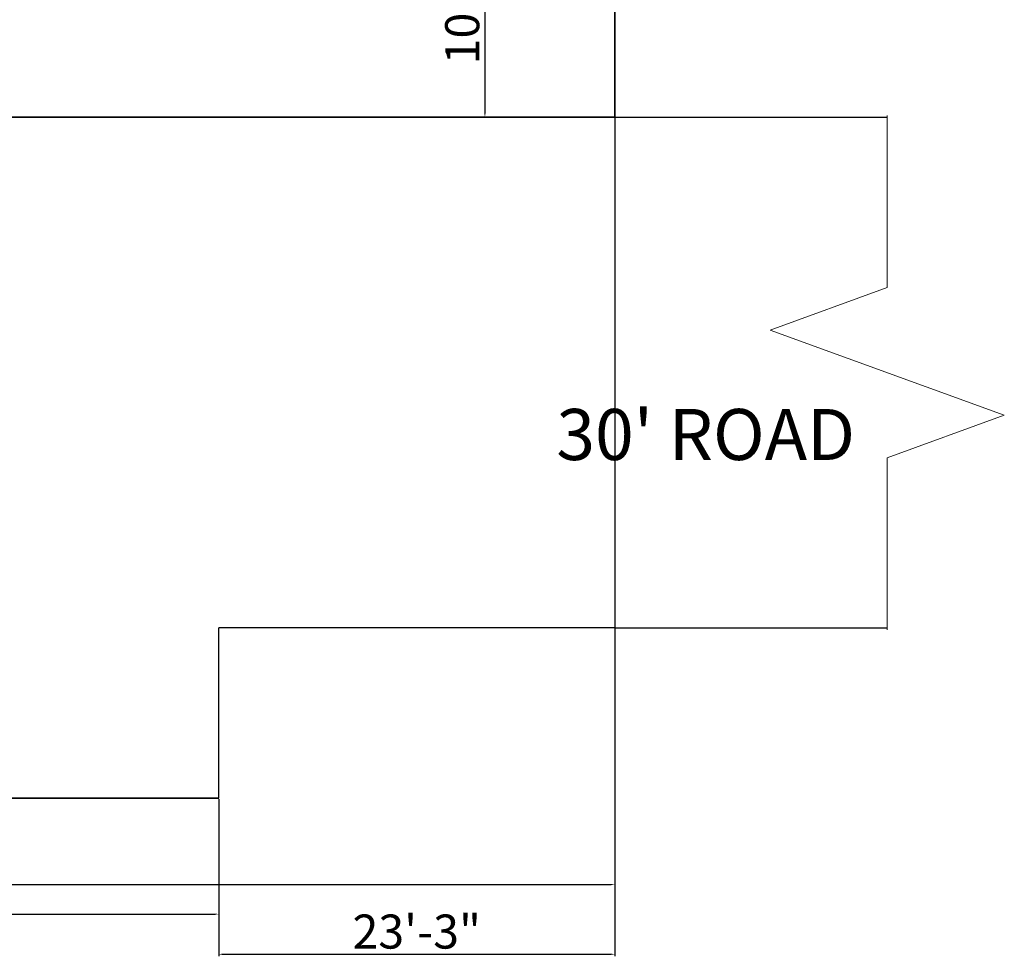
# Model space of a CAD drawing. Units: inches. Extents: x 2214 to 3937, y 762 to 2085.
# Tile 7 of 9: x 3243 to 3937, y 762 to 1424. Entities that reach past the tile are written whole.
import ezdxf

# ---------------------------------------------------------------- set-up
doc = ezdxf.new("R2010")
doc.units = ezdxf.units.IN
for name, color, linetype, lineweight in [('C-ANNO-DIMS', 2, 'Continuous', 18), ('C-ANNO-TEXT', 2, 'Continuous', 25), ('C-PROP', 3, 'Continuous', 35), ('C-ROAD', 2, 'Continuous', 25), ('C-ROAD-SYMB', 2, 'Continuous', 18)]:
    doc.layers.add(name, color=color, linetype=linetype, lineweight=lineweight)
doc.styles.get("Standard").update_dxf_attribs({"font": 'arial.ttf'})
doc.dimstyles.new('ISO-25', dxfattribs={"dimtxt": 10, "dimasz": 2.5, "dimexe": 1.25, "dimexo": 0.625, "dimtad": 1, "dimdec": 1, "dimlunit": 4, "dimtxsty": 'Standard', "dimcen": 2.5, "dimadec": 0, "dimazin": 0, "dimtfac": 1, "dimtdec": 1, "dimtmove": 0, "dimatfit": 3, "dimfxl": 1, "dimarcsym": 0})

# ---------------------------------------------------------------- blocks, each defined once
blk = doc.blocks.new('*D14')
at = {"layer": 'C-ANNO-DIMS', "color": 0, "lineweight": -2, "ltscale": 0.3, "transparency": 16777216}
for p, q in [((2582.56, 1354.59), (2582.56, 813.24)), ((3662.56, 1354.59), (3662.56, 813.24)), ((2585.06, 814.49), (3660.06, 814.49))]:
    blk.add_line(p, q, dxfattribs=at)
at = {"layer": 'C-ANNO-DIMS', "color": 0, "ltscale": 0.3, "transparency": 16777216}
for points in [[(2585.06, 814.91), (2585.06, 814.08), (2582.56, 814.49)], [(3660.06, 814.91), (3660.06, 814.08), (3662.56, 814.49)]]:
    blk.add_solid(points, dxfattribs=at)
at = {"layer": 'Defpoints', "color": 0, "ltscale": 0.3, "transparency": 16777216}
for p in [(2582.56, 1355.22), (3662.56, 1355.22), (3662.56, 814.49)]:
    blk.add_point(p, dxfattribs=at)
at = {"layer": 'C-ANNO-DIMS', "color": 0, "ltscale": 0.3, "transparency": 16777216, "insert": (3122.56, 827.37), "char_height": 24, "attachment_point": 5}
blk.add_mtext("90'", dxfattribs=at)
blk = doc.blocks.new('*D16')
at = {"layer": 'C-ANNO-DIMS', "color": 0, "lineweight": -2, "ltscale": 0.3, "transparency": 16777216}
for p, q in [((3662.56, 1354.59), (3662.56, 764.03)), ((3383.56, 874.59), (3383.56, 764.03)), ((3386.06, 765.28), (3660.06, 765.28))]:
    blk.add_line(p, q, dxfattribs=at)
at = {"layer": 'C-ANNO-DIMS', "color": 0, "ltscale": 0.3, "transparency": 16777216}
for points in [[(3386.06, 765.69), (3386.06, 764.86), (3383.56, 765.28)], [(3660.06, 765.69), (3660.06, 764.86), (3662.56, 765.28)]]:
    blk.add_solid(points, dxfattribs=at)
at = {"layer": 'Defpoints', "color": 0, "ltscale": 0.3, "transparency": 16777216}
for p in [(3662.56, 1355.22), (3383.56, 875.22), (3662.56, 765.28)]:
    blk.add_point(p, dxfattribs=at)
at = {"layer": 'C-ANNO-DIMS', "color": 0, "ltscale": 0.3, "transparency": 16777216, "insert": (3523.06, 778.16), "char_height": 24, "attachment_point": 5}
blk.add_mtext('23\'-3"', dxfattribs=at)
blk = doc.blocks.new('*D23')
at = {"layer": 'C-ANNO-DIMS', "color": 0, "lineweight": -2, "ltscale": 0.3, "transparency": 16777216}
for p, q in [((3571.06, 1472.72), (3571.06, 1357.72)), ((3571.68, 1475.22), (3572.31, 1475.22)), ((3571.68, 1355.22), (3572.31, 1355.22))]:
    blk.add_line(p, q, dxfattribs=at)
at = {"layer": 'C-ANNO-DIMS', "color": 0, "ltscale": 0.3, "transparency": 16777216}
for points in [[(3570.64, 1472.72), (3571.47, 1472.72), (3571.06, 1475.22)], [(3570.64, 1357.72), (3571.47, 1357.72), (3571.06, 1355.22)]]:
    blk.add_solid(points, dxfattribs=at)
at = {"layer": 'Defpoints', "color": 0, "ltscale": 0.3, "transparency": 16777216}
for p in [(3571.06, 1475.22), (3571.06, 1355.22), (3571.06, 1355.22)]:
    blk.add_point(p, dxfattribs=at)
at = {"layer": 'C-ANNO-DIMS', "color": 0, "ltscale": 0.3, "transparency": 16777216, "insert": (3558.18, 1415.22), "char_height": 24, "attachment_point": 5, "rotation": 90}
blk.add_mtext("10'", dxfattribs=at)
blk = doc.blocks.new('ROAD-BREAK-30FT')
at = {"ltscale": 0.3}
blk.add_lwpolyline([(82.42, 362.5), (82.42, 241.25), (0, 211.25), (164.85, 151.25), (82.42, 121.25), (82.42, 0)], dxfattribs=at)
blk = doc.blocks.new('*D61')
at = {"layer": 'C-ANNO-DIMS', "color": 0, "lineweight": -2, "ltscale": 0.3, "transparency": 16777216}
for p, q in [((2906.56, 874.59), (2906.56, 792.32)), ((3383.56, 874.59), (3383.56, 792.32)), ((2909.06, 793.57), (3381.06, 793.57))]:
    blk.add_line(p, q, dxfattribs=at)
at = {"layer": 'C-ANNO-DIMS', "color": 0, "ltscale": 0.3, "transparency": 16777216}
for points in [[(2909.06, 793.99), (2909.06, 793.15), (2906.56, 793.57)], [(3381.06, 793.99), (3381.06, 793.15), (3383.56, 793.57)]]:
    blk.add_solid(points, dxfattribs=at)
at = {"layer": 'Defpoints', "color": 0, "ltscale": 0.3, "transparency": 16777216}
for p in [(2906.56, 875.22), (3383.56, 875.22), (3383.56, 793.57)]:
    blk.add_point(p, dxfattribs=at)
at = {"layer": 'C-ANNO-DIMS', "color": 0, "ltscale": 0.3, "transparency": 16777216, "insert": (3145.06, 799.3), "char_height": 10, "attachment_point": 5}
blk.add_mtext('39\'-9"', dxfattribs=at)

msp = doc.modelspace()

# ---------------------------------------------------------------- linework, layer by layer
at = {"layer": 'C-PROP'}
for p, q in [((3662.56, 2003.22), (3662.56, 1355.22)), ((3662.56, 1355.22), (2582.56, 1355.22))]:
    msp.add_line(p, q, dxfattribs=at)
at = {"layer": 'C-ROAD', "ltscale": 0.3}
for p, q in [((3662.56, 1355.22), (3734.56, 1355.22)), ((3734.56, 1355.22), (3854.56, 1355.22)), ((3383.56, 875.22), (3383.56, 995.22)), ((3662.56, 995.22), (3734.56, 995.22)), ((3734.56, 995.22), (3854.56, 995.22)), ((2906.56, 875.22), (3383.56, 875.22))]:
    msp.add_line(p, q, dxfattribs=at)
at = {"layer": 'C-ROAD'}
for p, q in [((3662.56, 995.22), (3383.56, 995.22)), ((3383.56, 875.22), (2906.56, 875.22))]:
    msp.add_line(p, q, dxfattribs=at)

# ---------------------------------------------------------------- block references
at = {"layer": 'C-ROAD-SYMB'}
msp.add_blockref('ROAD-BREAK-30FT', (3772.13, 993.97), dxfattribs=at)

# ---------------------------------------------------------------- texts
at = {"layer": 'C-ANNO-TEXT', "ltscale": 0.3}
msp.add_text("30' ROAD ", height=36, dxfattribs=at).set_placement((3621.4, 1113.59))

# ---------------------------------------------------------------- dimensions: what is measured, and where the dimension line sits
at = {"layer": 'C-ANNO-DIMS', "ltscale": 0.3}
dim = msp.add_linear_dim(base=(3571.06, 1355.22), p1=(3571.06, 1475.22), p2=(3571.06, 1355.22), angle=90, dimstyle='ISO-25', override={"dimtxt": 24, "dimclrd": 0, "dimclre": 0, "dimclrt": 0}, dxfattribs=at)
dim.commit()
dim.dimension.update_dxf_attribs({"geometry": '*D23', "text_midpoint": (3558.18, 1415.22)})
for base, p1, p2, override, picture, middle in [((3662.56, 814.49), (2582.56, 1355.22), (3662.56, 1355.22), {"dimtxt": 24, "dimclrd": 0, "dimclre": 0, "dimclrt": 0}, '*D14', (3122.56, 827.37)), ((3662.56, 765.28), (3383.56, 875.22), (3662.56, 1355.22), {"dimtxt": 24, "dimclrd": 0, "dimclre": 0, "dimclrt": 0}, '*D16', (3523.06, 778.16)), ((3383.56, 793.57), (2906.56, 875.22), (3383.56, 875.22), {"dimdec": 1, "dimlfac": 1, "dimrnd": 0, "dimzin": 1, "dimdsep": 46, "dimlunit": 4, "dimfrac": 2}, '*D61', (3145.06, 799.3))]:
    dim = msp.add_linear_dim(base=base, p1=p1, p2=p2, dimstyle='ISO-25', override=override, dxfattribs=at)
    dim.commit()
    dim.dimension.update_dxf_attribs({"geometry": picture, "text_midpoint": middle})

doc.saveas('drawing.dxf')
